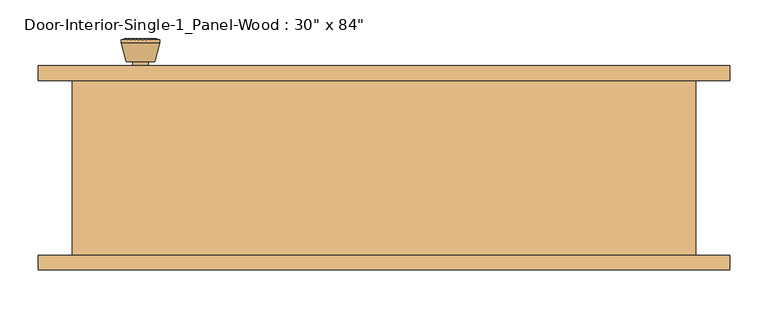
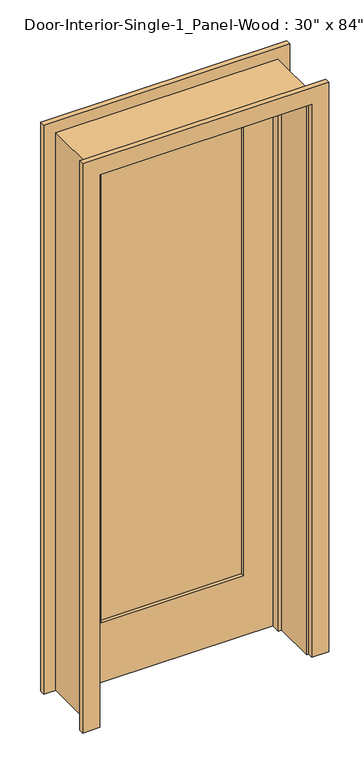
"""IFC4 building model written with IfcOpenShell, lengths in millimetres: door geometry."""

from ifc_helpers import new_model, si_unit, point, frame, frame_2d, origin, place, context, project, spatial, polyline, circle_curve, trimmed, segment, composite_curve, outline, extrude, faceted_brep, source, transform, mapped, element, save
from ifc_brep_helpers import plane_surface, cylinder_surface, revolved_surface, advanced_brep


def door_ac3c0746(model_context):
    return source(origin(), model_context, "Body", "SolidModel", [
        advanced_brep(
        [(-317.5, 70.2, 914.4), (-307.5, 70.2, 914.4), (-327.5, 70.2, 914.4), (-297.0241324, 21.2, 914.4), (-317.5, 21.2, 914.4), (-337.9758676, 21.2, 914.4), (-292.5, 23.0278681, 914.4), (-342.5, 23.0278681, 914.4), (-292.5, 26.4915463, 914.4), (-342.5, 26.4915463, 914.4), (-298.863764, 51.2, 914.4), (-336.136236, 51.2, 914.4), (-307.5, 51.2, 914.4), (-327.5, 51.2, 914.4)],
        [
            (0, 1),
            (1, 2, circle_curve(frame((-317.5, 70.2, 914.4), z_axis=(0.0, 1.0, 0.0), x_axis=(-1.0, 0.0, 0.0)), 10.0)),
            (2, 0),
            (2, 1, circle_curve(frame((-317.5, 70.2, 914.4), z_axis=(0.0, 1.0, 0.0), x_axis=(-1.0, 0.0, 0.0)), 10.0)),
            (3, 4),
            (4, 5),
            (5, 3, circle_curve(frame((-317.5, 21.2, 914.4), z_axis=(0.0, -1.0, 0.0), x_axis=(-1.0, 0.0, 0.0)), 20.4758676)),
            (3, 5, circle_curve(frame((-317.5, 21.2, 914.4), z_axis=(0.0, -1.0, 0.0), x_axis=(-1.0, 0.0, 0.0)), 20.4758676)),
            (6, 3),
            (5, 7),
            (7, 6, circle_curve(frame((-317.5, 23.0278681, 914.4), z_axis=(0.0, -1.0, 0.0), x_axis=(-1.0, 0.0, 0.0)), 25.0)),
            (6, 7, circle_curve(frame((-317.5, 23.0278681, 914.4), z_axis=(0.0, -1.0, 0.0), x_axis=(-1.0, 0.0, 0.0)), 25.0)),
            (8, 6),
            (7, 9),
            (9, 8, circle_curve(frame((-317.5, 26.4915463, 914.4), z_axis=(0.0, -1.0, 0.0), x_axis=(-1.0, 0.0, 0.0)), 25.0)),
            (8, 9, circle_curve(frame((-317.5, 26.4915463, 914.4), z_axis=(0.0, -1.0, 0.0), x_axis=(-1.0, 0.0, 0.0)), 25.0)),
            (10, 8),
            (9, 11),
            (11, 10, circle_curve(frame((-317.5, 51.2, 914.4), z_axis=(0.0, -1.0, 0.0), x_axis=(-1.0, 0.0, 0.0)), 18.636236)),
            (10, 11, circle_curve(frame((-317.5, 51.2, 914.4), z_axis=(0.0, -1.0, 0.0), x_axis=(-1.0, 0.0, 0.0)), 18.636236)),
            (12, 10),
            (11, 13),
            (13, 12, circle_curve(frame((-317.5, 51.2, 914.4), z_axis=(0.0, -1.0, 0.0), x_axis=(-1.0, 0.0, 0.0)), 10.0)),
            (12, 13, circle_curve(frame((-317.5, 51.2, 914.4), z_axis=(0.0, -1.0, 0.0), x_axis=(-1.0, 0.0, 0.0)), 10.0)),
            (1, 12),
            (13, 2),
        ],
        [
            plane_surface(frame((-317.5, 70.2, 914.4), z_axis=(0.0, 1.0, 0.0), x_axis=(-1.0, 0.0, 0.0))),
            plane_surface(frame((-317.5, 21.2, 914.4), z_axis=(0.0, -1.0, 0.0), x_axis=(-1.0, 0.0, 0.0))),
            revolved_surface(polyline([(-337.9758676, 21.2, 914.4), (-342.5, 23.0278681, 914.4)]), (-317.5, 70.2, 914.4), (0.0, 1.0, 0.0)),
            cylinder_surface(frame((-317.5, 70.2, 914.4), z_axis=(0.0, 1.0, 0.0), x_axis=(-1.0, 0.0, 0.0)), 25.0),
            revolved_surface(polyline([(-342.5, 26.4915463, 914.4), (-336.136236, 51.2, 914.4)]), (-317.5, 70.2, 914.4), (0.0, 1.0, 0.0)),
            plane_surface(frame((-317.5, 51.2, 914.4), z_axis=(0.0, 1.0, 0.0), x_axis=(-1.0, 0.0, 0.0))),
            cylinder_surface(frame((-317.5, 70.2, 914.4), z_axis=(0.0, 1.0, 0.0), x_axis=(-1.0, 0.0, 0.0)), 10.0),
        ],
        [
            (0, [[1, 2, 3]]),
            (0, [[-3, 4, -1]]),
            (1, [[5, 6, 7]]),
            (1, [[-6, -5, 8]]),
            (2, [[9, -7, 10, 11]]),
            (2, [[-10, -8, -9, 12]]),
            (3, [[13, -11, 14, 15]]),
            (3, [[-14, -12, -13, 16]]),
            (4, [[17, -15, 18, 19]]),
            (4, [[-18, -16, -17, 20]]),
            (5, [[21, -19, 22, 23]]),
            (5, [[-22, -20, -21, 24]]),
            (6, [[25, -23, 26, -2]]),
            (6, [[-26, -24, -25, -4]]),
        ],
    ),
        extrude(outline(composite_curve([segment(trimmed(circle_curve(frame_2d((914.4, -317.5)), 30.0), [point((914.4, -347.5))], [point((914.4, -287.5))], False, "CARTESIAN"), True, "CONTINUOUS"), segment(trimmed(circle_curve(frame_2d((914.4, -317.5)), 30.0), [point((914.4, -287.5))], [point((914.4, -347.5))], False, "CARTESIAN"), True, "CONTINUOUS")], self_intersect=False)), frame((0.0, 70.2, 0.0), z_axis=(0.0, 1.0, 0.0), x_axis=(0.0, 0.0, 1.0)), (0.0, 0.0, 1.0), 6.0),
        advanced_brep(
        [(-317.5, 117.125, 914.4), (-327.5, 117.125, 914.4), (-307.5, 117.125, 914.4), (-297.0241324, 166.125, 914.4), (-337.9758676, 166.125, 914.4), (-317.5, 166.125, 914.4), (-292.5, 164.2971319, 914.4), (-342.5, 164.2971319, 914.4), (-292.5, 160.8334537, 914.4), (-342.5, 160.8334537, 914.4), (-298.863764, 136.125, 914.4), (-336.136236, 136.125, 914.4), (-307.5, 136.125, 914.4), (-327.5, 136.125, 914.4)],
        [
            (0, 1),
            (1, 2, circle_curve(frame((-317.5, 117.125, 914.4), z_axis=(0.0, -1.0, 0.0), x_axis=(-1.0, 0.0, 0.0)), 10.0)),
            (2, 0),
            (2, 1, circle_curve(frame((-317.5, 117.125, 914.4), z_axis=(0.0, -1.0, 0.0), x_axis=(-1.0, 0.0, 0.0)), 10.0)),
            (3, 4, circle_curve(frame((-317.5, 166.125, 914.4), z_axis=(0.0, 1.0, 0.0), x_axis=(-1.0, 0.0, 0.0)), 20.4758676)),
            (4, 5),
            (5, 3),
            (4, 3, circle_curve(frame((-317.5, 166.125, 914.4), z_axis=(0.0, 1.0, 0.0), x_axis=(-1.0, 0.0, 0.0)), 20.4758676)),
            (6, 7, circle_curve(frame((-317.5, 164.2971319, 914.4), z_axis=(0.0, 1.0, 0.0), x_axis=(-1.0, 0.0, 0.0)), 25.0)),
            (7, 4),
            (3, 6),
            (7, 6, circle_curve(frame((-317.5, 164.2971319, 914.4), z_axis=(0.0, 1.0, 0.0), x_axis=(-1.0, 0.0, 0.0)), 25.0)),
            (8, 9, circle_curve(frame((-317.5, 160.8334537, 914.4), z_axis=(0.0, 1.0, 0.0), x_axis=(-1.0, 0.0, 0.0)), 25.0)),
            (9, 7),
            (6, 8),
            (9, 8, circle_curve(frame((-317.5, 160.8334537, 914.4), z_axis=(0.0, 1.0, 0.0), x_axis=(-1.0, 0.0, 0.0)), 25.0)),
            (10, 11, circle_curve(frame((-317.5, 136.125, 914.4), z_axis=(0.0, 1.0, 0.0), x_axis=(-1.0, 0.0, 0.0)), 18.636236)),
            (11, 9),
            (8, 10),
            (11, 10, circle_curve(frame((-317.5, 136.125, 914.4), z_axis=(0.0, 1.0, 0.0), x_axis=(-1.0, 0.0, 0.0)), 18.636236)),
            (12, 13, circle_curve(frame((-317.5, 136.125, 914.4), z_axis=(0.0, 1.0, 0.0), x_axis=(-1.0, 0.0, 0.0)), 10.0)),
            (13, 11),
            (10, 12),
            (13, 12, circle_curve(frame((-317.5, 136.125, 914.4), z_axis=(0.0, 1.0, 0.0), x_axis=(-1.0, 0.0, 0.0)), 10.0)),
            (1, 13),
            (12, 2),
        ],
        [
            plane_surface(frame((-317.5, 117.125, 914.4), z_axis=(0.0, -1.0, 0.0), x_axis=(-1.0, 0.0, 0.0))),
            plane_surface(frame((-317.5, 166.125, 914.4), z_axis=(0.0, 1.0, 0.0), x_axis=(-1.0, 0.0, 0.0))),
            revolved_surface(polyline([(-337.9758676, 166.125, 914.4), (-342.5, 164.2971319, 914.4)]), (-317.5, 117.125, 914.4), (0.0, -1.0, 0.0)),
            cylinder_surface(frame((-317.5, 117.125, 914.4), z_axis=(0.0, -1.0, 0.0), x_axis=(-1.0, 0.0, 0.0)), 25.0),
            revolved_surface(polyline([(-342.5, 160.8334537, 914.4), (-336.136236, 136.125, 914.4)]), (-317.5, 117.125, 914.4), (0.0, -1.0, 0.0)),
            plane_surface(frame((-317.5, 136.125, 914.4), z_axis=(0.0, -1.0, 0.0), x_axis=(-1.0, 0.0, 0.0))),
            cylinder_surface(frame((-317.5, 117.125, 914.4), z_axis=(0.0, -1.0, 0.0), x_axis=(-1.0, 0.0, 0.0)), 10.0),
        ],
        [
            (0, [[1, 2, 3]]),
            (0, [[-3, 4, -1]]),
            (1, [[5, 6, 7]]),
            (1, [[8, -7, -6]]),
            (2, [[9, 10, -5, 11]]),
            (2, [[12, -11, -8, -10]]),
            (3, [[13, 14, -9, 15]]),
            (3, [[16, -15, -12, -14]]),
            (4, [[17, 18, -13, 19]]),
            (4, [[20, -19, -16, -18]]),
            (5, [[21, 22, -17, 23]]),
            (5, [[24, -23, -20, -22]]),
            (6, [[-2, 25, -21, 26]]),
            (6, [[-4, -26, -24, -25]]),
        ],
    ),
        extrude(outline(composite_curve([segment(trimmed(circle_curve(frame_2d((914.4, -317.5)), 30.0), [point((914.4, -347.5))], [point((914.4, -287.5))], False, "CARTESIAN"), True, "CONTINUOUS"), segment(trimmed(circle_curve(frame_2d((914.4, -317.5)), 30.0), [point((914.4, -287.5))], [point((914.4, -347.5))], False, "CARTESIAN"), True, "CONTINUOUS")], self_intersect=False)), frame((0.0, 111.125, 0.0), z_axis=(0.0, 1.0, 0.0), x_axis=(0.0, 0.0, 1.0)), (0.0, 0.0, 1.0), 6.0),
        faceted_brep([(406.4, 111.125, 0.0), (406.4, -117.475, 0.0), (381.0, -117.475, 0.0), (381.0, 41.275, 0.0), (368.3, 41.275, 0.0), (368.3, 76.2, 0.0), (381.0, 76.2, 0.0), (381.0, 111.125, 0.0), (406.4, 111.125, 2159.0), (406.4, -117.475, 2159.0), (-406.4, -117.475, 2159.0), (-406.4, -117.475, 0.0), (-381.0, -117.475, 0.0), (-381.0, -117.475, 2133.6), (381.0, -117.475, 2133.6), (381.0, 41.275, 2133.6), (-381.0, 41.275, 2133.6), (-381.0, 41.275, 0.0), (-368.3, 41.275, 0.0), (-368.3, 41.275, 2120.9), (368.3, 41.275, 2120.9), (368.3, 76.2, 2120.9), (-368.3, 76.2, 2120.9), (-368.3, 76.2, 0.0), (-381.0, 76.2, 0.0), (-381.0, 76.2, 2133.6), (381.0, 76.2, 2133.6), (381.0, 111.125, 2133.6), (-381.0, 111.125, 2133.6), (-381.0, 111.125, 0.0), (-406.4, 111.125, 0.0), (-406.4, 111.125, 2159.0)], [[[0, 1, 2, 3, 4, 5, 6, 7]], [[1, 0, 8, 9]], [[2, 1, 9, 10, 11, 12, 13, 14]], [[3, 2, 14, 15]], [[4, 3, 15, 16, 17, 18, 19, 20]], [[5, 4, 20, 21]], [[6, 5, 21, 22, 23, 24, 25, 26]], [[7, 6, 26, 27]], [[0, 7, 27, 28, 29, 30, 31, 8]], [[9, 8, 31, 10]], [[15, 14, 13, 16]], [[21, 20, 19, 22]], [[27, 26, 25, 28]], [[30, 29, 24, 23, 18, 17, 12, 11]], [[10, 31, 30, 11]], [[16, 13, 12, 17]], [[22, 19, 18, 23]], [[28, 25, 24, 29]]]),
        extrude(outline(polyline([(2133.6, -381.0), (0.0, -381.0), (0.0, 381.0), (2133.6, 381.0), (2133.6, -381.0)]), holes=[polyline([(2014.5375, -260.35), (2014.5375, 260.35), (231.775, 260.35), (231.775, -260.35), (2014.5375, -260.35)])]), frame((0.0, 76.2, 0.0), z_axis=(0.0, 1.0, 0.0), x_axis=(0.0, 0.0, 1.0)), (0.0, 0.0, 1.0), 34.925),
        extrude(outline(polyline([(260.35, 87.8416667), (-260.35, 87.8416667), (-260.35, 99.4833333), (260.35, 99.4833333), (260.35, 87.8416667)])), frame((0.0, 0.0, 231.775), z_axis=(0.0, 0.0, 1.0), x_axis=(1.0, 0.0, 0.0)), (0.0, 0.0, 1.0), 1782.7625),
        extrude(outline(polyline([(0.0, 387.35), (0.0, 450.85), (2203.45, 450.85), (2203.45, -450.85), (0.0, -450.85), (0.0, -387.35), (2139.95, -387.35), (2139.95, 387.35), (0.0, 387.35)])), frame((0.0, 111.125, 0.0), z_axis=(0.0, 1.0, 0.0), x_axis=(0.0, 0.0, 1.0)), (0.0, 0.0, 1.0), 19.05),
        extrude(outline(polyline([(0.0, 387.35), (0.0, 450.85), (2203.45, 450.85), (2203.45, -450.85), (0.0, -450.85), (0.0, -387.35), (2139.95, -387.35), (2139.95, 387.35), (0.0, 387.35)])), frame((0.0, -136.525, 0.0), z_axis=(0.0, 1.0, 0.0), x_axis=(0.0, 0.0, 1.0)), (0.0, 0.0, 1.0), 19.05),
    ])


if __name__ == "__main__":
    model = new_model("IFC4")
    model_context = context("Model", 3, world=origin())
    ifc_project = project(units=[si_unit("LENGTHUNIT", "METRE", prefix="MILLI")], contexts=[model_context])
    site = spatial("IfcSite", under=ifc_project)
    building = spatial("IfcBuilding", under=site)
    placement = place(None, origin())
    door_shape = door_ac3c0746(model_context)
    element("IfcDoor", 1, ObjectType="Door-Interior-Single-1_Panel-Wood : 30\" x 84\"", at=placement, inside=building, context=model_context, shape_type="MappedRepresentation", body=[
        mapped(door_shape, transform((0.0, 0.0, 0.0), x_axis=(1.0, 0.0, 0.0), y_axis=(0.0, 1.0, 0.0), z_axis=(0.0, 0.0, 1.0))),
    ])
    save(model, "model.ifc")

# Revit data of these elements
# Type "Door-Interior-Single-1_Panel-Wood : 30\" x 84\""
#   Type Mark = "11"
#   Assembly Code = "C1020300"
#   Analytic Construction = "Wooden"
#   Top Rail = 0' - 4 11/16"
#   Thickness = 0' - 1 3/8"
#   Thermal Resistance (R) = 2.5876 (h·ft²·°F)/BTU
#   Swing Angle [instance default] = 90.00°
#   Stiles = 0' - 4 3/4"
#   Rough Width = 2' - 8"
#   Rough Height = 7' - 1"
#   Height = 7' - 0"
#   Width = 2' - 6"
#   Heat Transfer Coefficient (U) = 0.3865 BTU/(h·ft²·°F)
#   Bottom Rail = 0' - 9 1/8"
#   Trim Material = Cherry
#   Panel Material = Cherry
#   Frame Material = Cherry
#   Door Handle Material = Aluminum
#   Visual Light Transmittance = 0
#   Solar Heat Gain Coefficient = 0
#   Wall Closure = (empty or 0)
#   Function = (empty or 0)
# Element 1 (IfcDoor, "Door-Interior-Single-1_Panel-Wood : 30\" x 84\"")
#   Materials on its faces: "Cherry", "Aluminum"
# Materials
#   "Cherry": class "Wood", colour RGB 226 177 128, transparency 0, Description = "Prunus Serotina", Cost = 0
#   "Aluminum": class "Metal", colour RGB 247 247 247, transparency 0, Description = "Aluminum 6061", Cost = 0
